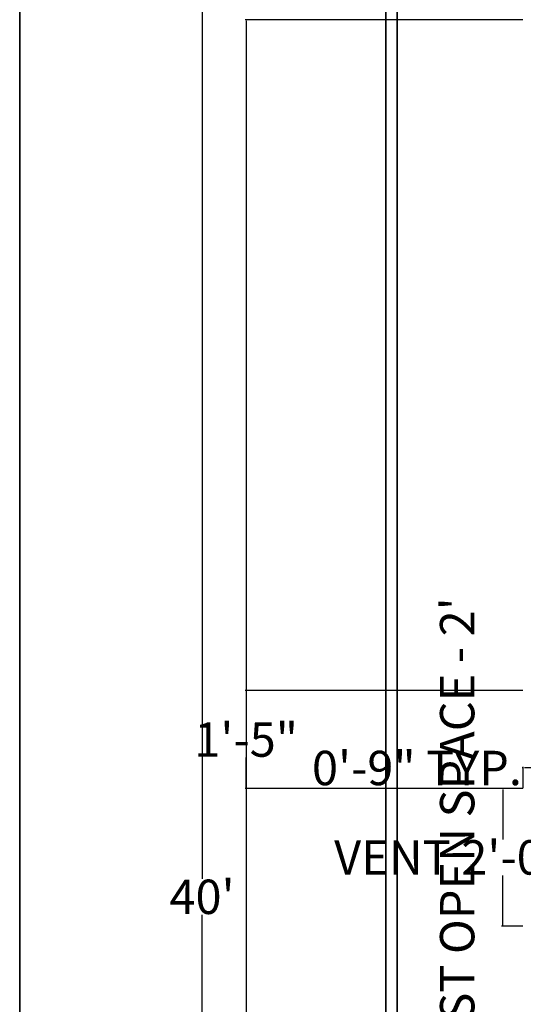
# Model space of a CAD drawing. Units: inches. Extents: x 1601 to 2080, y 5000 to 5589.
# Tile 7 of 11: x 1601 to 1688, y 5259 to 5431. Entities that reach past the tile are written whole.
import ezdxf

# ---------------------------------------------------------------- set-up
doc = ezdxf.new("R2010")
doc.units = ezdxf.units.IN
doc.header["$MEASUREMENT"] = 0
for name, color, linetype, lineweight in [('A-ANNO-DIMS', 2, 'Continuous', 18), ('A-ANNO-TTLB', 7, 'Continuous', 35), ('A-AREA-IDEN', 7, 'Continuous', 25), ('C-PROP', 7, 'Continuous', 35)]:
    doc.layers.add(name, color=color, linetype=linetype, lineweight=lineweight)
doc.styles.get("Standard").update_dxf_attribs({"font": 'arial.ttf'})
doc.dimstyles.get("Standard").update_dxf_attribs({"dimtxt": 6, "dimasz": 0.18, "dimexe": 0.18, "dimexo": 0.0625, "dimgap": 0.09, "dimtad": 0, "dimtih": 1, "dimtoh": 1, "dimdec": 1, "dimzin": 0, "dimdsep": 46, "dimlunit": 3, "dimtxsty": 'Standard', "dimcen": 0.09, "dimadec": 0, "dimazin": 0, "dimtfac": 1, "dimtdec": 1, "dimtofl": 0, "dimtmove": 0, "dimatfit": 3, "dimfxl": 1, "dimtolj": 1, "dimtzin": 0, "dimarcsym": 0})

# ---------------------------------------------------------------- blocks, each defined once
blk = doc.blocks.new('*D4')
at = {"layer": 'A-ANNO-DIMS', "color": 0, "lineweight": -2, "transparency": 16777216}
for p, q in [((1664.35, 5509.2), (1632.18, 5509.2)), ((1632.36, 5509.02), (1632.36, 5281.35)), ((1632.36, 5047.39), (1632.36, 5275.05)), ((1664.35, 5047.21), (1632.18, 5047.21))]:
    blk.add_line(p, q, dxfattribs=at)
at = {"layer": 'A-ANNO-DIMS', "color": 0, "transparency": 16777216}
for points in [[(1632.33, 5509.02), (1632.39, 5509.02), (1632.36, 5509.2)], [(1632.33, 5047.39), (1632.39, 5047.39), (1632.36, 5047.21)]]:
    blk.add_solid(points, dxfattribs=at)
at = {"layer": 'Defpoints', "color": 0, "transparency": 16777216}
for p in [(1664.41, 5509.2), (1632.36, 5047.21), (1664.41, 5047.21)]:
    blk.add_point(p, dxfattribs=at)
at = {"layer": 'A-ANNO-DIMS', "color": 0, "transparency": 16777216, "insert": (1632.36, 5278.2), "char_height": 6, "attachment_point": 5}
blk.add_mtext("\\A1;40'", dxfattribs=at)
blk = doc.blocks.new('*D31')
at = {"layer": 'A-ANNO-DIMS', "color": 0, "lineweight": -2, "transparency": 16777216}
for p, q in [((1688.35, 5297.07), (1684.63, 5297.07)), ((1684.81, 5296.89), (1684.81, 5288.22)), ((1684.81, 5273.25), (1684.81, 5281.92)), ((1688.35, 5273.07), (1684.63, 5273.07))]:
    blk.add_line(p, q, dxfattribs=at)
at = {"layer": 'A-ANNO-DIMS', "color": 0, "transparency": 16777216}
for points in [[(1684.78, 5296.89), (1684.84, 5296.89), (1684.81, 5297.07)], [(1684.78, 5273.25), (1684.84, 5273.25), (1684.81, 5273.07)]]:
    blk.add_solid(points, dxfattribs=at)
at = {"layer": 'Defpoints', "color": 0, "transparency": 16777216}
for p in [(1688.41, 5297.07), (1684.81, 5273.07), (1688.41, 5273.07)]:
    blk.add_point(p, dxfattribs=at)
at = {"layer": 'A-ANNO-DIMS', "color": 0, "transparency": 16777216, "insert": (1684.81, 5285.07), "char_height": 6, "attachment_point": 5}
blk.add_mtext('\\A1;VENT 2\'-0" TYP.', dxfattribs=at)
blk = doc.blocks.new('*D32')
at = {"layer": 'A-ANNO-DIMS', "color": 0, "lineweight": -2, "transparency": 16777216}
for p, q in [((1688.41, 5300.67), (1688.23, 5300.67)), ((1688.41, 5297.13), (1688.41, 5300.85)), ((1697.23, 5300.67), (1688.59, 5300.67)), ((1697.41, 5297.13), (1697.41, 5300.85))]:
    blk.add_line(p, q, dxfattribs=at)
at = {"layer": 'A-ANNO-DIMS', "color": 0, "transparency": 16777216}
for points in [[(1688.59, 5300.7), (1688.59, 5300.64), (1688.41, 5300.67)], [(1697.23, 5300.7), (1697.23, 5300.64), (1697.41, 5300.67)]]:
    blk.add_solid(points, dxfattribs=at)
at = {"layer": 'Defpoints', "color": 0, "transparency": 16777216}
for p in [(1688.41, 5300.67), (1688.41, 5297.07), (1697.41, 5297.07)]:
    blk.add_point(p, dxfattribs=at)
at = {"layer": 'A-ANNO-DIMS', "color": 0, "transparency": 16777216, "insert": (1669.85, 5300.67), "char_height": 6, "attachment_point": 5}
blk.add_mtext('\\A1;0\'-9" TYP.', dxfattribs=at)
blk = doc.blocks.new('*D38')
at = {"layer": 'A-ANNO-DIMS', "color": 0, "lineweight": -2, "transparency": 16777216}
for p, q in [((1688.35, 5431.2), (1639.88, 5431.2)), ((1640.06, 5431.02), (1640.06, 5253.64)), ((1640.06, 5069.88), (1640.06, 5247.25)), ((1688.35, 5069.7), (1639.88, 5069.7))]:
    blk.add_line(p, q, dxfattribs=at)
at = {"layer": 'A-ANNO-DIMS', "color": 0, "transparency": 16777216}
for points in [[(1640.03, 5431.02), (1640.09, 5431.02), (1640.06, 5431.2)], [(1640.03, 5069.88), (1640.09, 5069.88), (1640.06, 5069.7)]]:
    blk.add_solid(points, dxfattribs=at)
at = {"layer": 'Defpoints', "color": 0, "transparency": 16777216}
for p in [(1640.06, 5431.2), (1688.41, 5431.2), (1688.41, 5069.7)]:
    blk.add_point(p, dxfattribs=at)
at = {"layer": 'A-ANNO-DIMS', "color": 0, "transparency": 16777216, "insert": (1640.06, 5250.45), "char_height": 6, "attachment_point": 5}
blk.add_mtext('\\A1;30\'-1 1/2"', dxfattribs=at)
blk = doc.blocks.new('*D53')
at = {"layer": 'A-ANNO-DIMS', "color": 0, "lineweight": -2, "transparency": 16777216}
for p, q in [((1688.35, 5314.2), (1639.88, 5314.2)), ((1640.06, 5314.02), (1640.06, 5308.79)), ((1640.06, 5297.25), (1640.06, 5302.48)), ((1688.35, 5297.07), (1639.88, 5297.07))]:
    blk.add_line(p, q, dxfattribs=at)
at = {"layer": 'A-ANNO-DIMS', "color": 0, "transparency": 16777216}
for points in [[(1640.03, 5314.02), (1640.09, 5314.02), (1640.06, 5314.2)], [(1640.03, 5297.25), (1640.09, 5297.25), (1640.06, 5297.07)]]:
    blk.add_solid(points, dxfattribs=at)
at = {"layer": 'Defpoints', "color": 0, "transparency": 16777216}
for p in [(1640.06, 5314.2), (1688.41, 5314.2), (1688.41, 5297.07)]:
    blk.add_point(p, dxfattribs=at)
at = {"layer": 'A-ANNO-DIMS', "color": 0, "transparency": 16777216, "insert": (1640.06, 5305.63), "char_height": 6, "attachment_point": 5}
blk.add_mtext('\\A1;1\'-5"', dxfattribs=at)

msp = doc.modelspace()

# ---------------------------------------------------------------- linework, layer by layer
at = {"layer": 'A-ANNO-TTLB'}
msp.add_lwpolyline([(1600.55, 5589.45), (2079.72, 5589.45), (2079.72, 4999.95), (1600.55, 4999.95)], close=True, dxfattribs=at)
at = {"layer": 'C-PROP'}
for p, q in [((1664.41, 5509.2), (1664.41, 5047.21)), ((1666.41, 5507.2), (1666.41, 5069.7))]:
    msp.add_line(p, q, dxfattribs=at)

# ---------------------------------------------------------------- texts
at = {"layer": 'A-AREA-IDEN', "insert": (1673.87, 5244.59), "char_height": 6, "attachment_point": 1, "rotation": 90}
msp.add_mtext_dynamic_manual_height_columns("WEST OPEN SPACE - 2'", width=126.5515, gutter_width=30, heights=[0], dxfattribs=at)

# ---------------------------------------------------------------- dimensions: what is measured, and where the dimension line sits
at = {"layer": 'A-ANNO-DIMS'}
for base, p1, p2, angle, text, override, picture, middle in [((1632.36, 5047.21), (1664.41, 5509.2), (1664.41, 5047.21), 90, "40'", {"dimclrd": 0, "dimclre": 0, "dimclrt": 0}, '*D4', (1632.36, 5278.2)), ((1688.41, 5300.67), (1697.41, 5297.07), (1688.41, 5297.07), 180, '<> TYP.', {"dimdec": 1, "dimlfac": 1, "dimrnd": 0, "dimzin": 1, "dimdsep": 46, "dimlunit": 4, "dimfrac": 2}, '*D32', (1669.85, 5300.67)), ((1684.81, 5273.07), (1688.41, 5297.07), (1688.41, 5273.07), 270, 'VENT <> TYP.', {"dimdec": 1, "dimlfac": 1, "dimrnd": 0, "dimzin": 1, "dimdsep": 46, "dimlunit": 4, "dimfrac": 2}, '*D31', (1684.81, 5285.07))]:
    dim = msp.add_linear_dim(base=base, p1=p1, p2=p2, angle=angle, text=text, dimstyle='Standard', override=override, dxfattribs=at)
    dim.commit()
    dim.dimension.update_dxf_attribs({"geometry": picture, "text_midpoint": middle})
for base, p1, p2, picture, middle in [((1640.06, 5431.2), (1688.41, 5069.7), (1688.41, 5431.2), '*D38', (1640.06, 5250.45)), ((1640.06, 5314.2), (1688.41, 5297.07), (1688.41, 5314.2), '*D53', (1640.06, 5305.63))]:
    dim = msp.add_linear_dim(base=base, p1=p1, p2=p2, angle=90, dimstyle='Standard', override={"dimdec": 1, "dimlfac": 1, "dimrnd": 0, "dimzin": 1, "dimdsep": 46, "dimlunit": 4, "dimfrac": 2}, dxfattribs=at)
    dim.commit()
    dim.dimension.update_dxf_attribs({"geometry": picture, "text_midpoint": middle})

doc.saveas('drawing.dxf')
